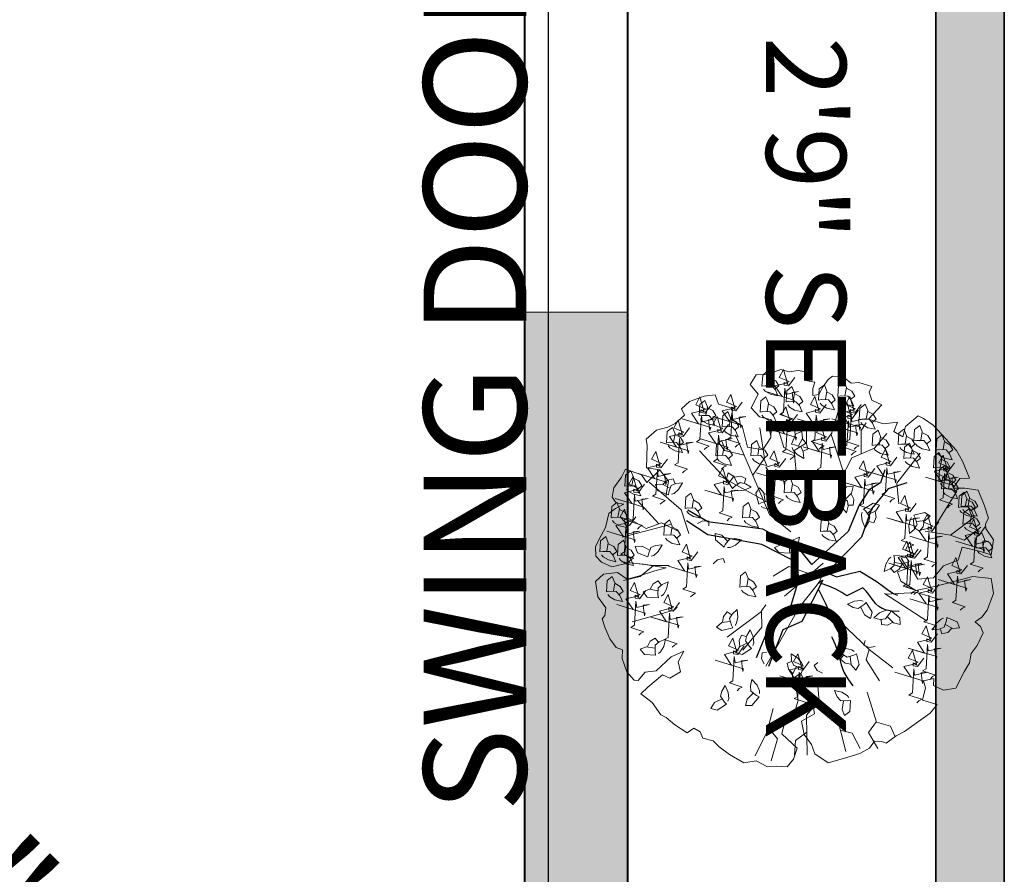
# Model space of a CAD drawing. Units: inches. Extents: x 2337 to 3570, y 1258 to 1938.
# Tile 26 of 30: x 3382 to 3468, y 1598 to 1673. Entities that reach past the tile are written whole.
import ezdxf

# ---------------------------------------------------------------- set-up
doc = ezdxf.new("R2010")
doc.units = ezdxf.units.IN
for name, color, linetype, lineweight in [('A-ANNO-DIMS', 2, 'Continuous', 18), ('A-ANNO-TEXT', 7, 'Continuous', 18), ('A-GLAZ', 4, 'Continuous', 18), ('A-WALL', 7, 'Continuous', 40), ('ARBOL', 74, 'Continuous', 13), ('C-PROP', 7, 'Continuous', 35)]:
    doc.layers.add(name, color=color, linetype=linetype, lineweight=lineweight)
doc.layers.add('A-WALL-PATT', color=18, linetype='Continuous', lineweight=13, true_color=0x000000)
doc.layers.add('C-PROP-PATT', color=251, linetype='Continuous', lineweight=13, true_color=0x636466)
doc.layers.add('TALLO', color=36, linetype='Continuous')
doc.styles.get("Standard").update_dxf_attribs({"font": 'arial.ttf'})
doc.dimstyles.new('ISO-25', dxfattribs={"dimtxt": 9, "dimasz": 2.5, "dimexe": 1.25, "dimexo": 0.625, "dimtad": 1, "dimdec": 1, "dimlunit": 3, "dimtxsty": 'Standard', "dimcen": 2.5, "dimadec": 0, "dimazin": 0, "dimtfac": 1, "dimtdec": 1, "dimtmove": 0, "dimatfit": 3, "dimfxl": 1, "dimarcsym": 0})

# ---------------------------------------------------------------- blocks, each defined once
blk = doc.blocks.new('fresno')
at = {"layer": 'ARBOL'}
for p, q in [((2.96, 0.991), (3.575, 1.984)), ((-3.638, 1.194), (-4.164, 1.76)), ((-1.151, -0.932), (-1.99, -1.556)), ((-0.974, -3.757), (-1.31, -4.423))]:
    blk.add_line(p, q, dxfattribs=at)
blk.add_lwpolyline([(0.823, 4.745), (0.566, 4.764), (0.459, 4.687), (0.336, 4.518), (0.233, 4.322), (0.087, 4.298), (0.091, 4.464), (0.14, 4.621), (-0.09, 4.659), (-0.033, 4.863), (-0.264, 4.901), (-0.483, 4.866), (-0.686, 4.924), (-1.021, 4.801), (-1.288, 4.8), (-1.431, 4.563), (-1.234, 4.327), (-1.406, 4), (-1.205, 3.778), (-0.909, 3.705), (-0.931, 3.283), (-1.122, 2.983), (-1.491, 3.043), (-1.619, 3.562), (-1.9, 3.727), (-1.851, 3.982), (-2.197, 4.084), (-2.278, 4.31), (-2.543, 4.283), (-2.896, 4.152), (-3.091, 3.971), (-3.022, 3.817), (-3.244, 3.617), (-3.424, 3.528), (-3.697, 3.455), (-3.946, 3.236), (-3.922, 3.09), (-3.94, 2.548), (-3.617, 2.495), (-3.927, 2.19), (-4.062, 2.379), (-4.443, 2.512), (-4.546, 2.316), (-4.73, 2.062), (-4.767, 1.832), (-4.671, 1.698), (-4.486, 1.667), (-4.693, 1.559), (-4.854, 1.444), (-4.934, 1.102), (-5.037, 0.905), (-5.175, 0.644), (-5.166, 0.406), (-5.024, 0.264), (-4.781, 0.153), (-4.363, 0.249), (-4.014, 0.215), (-3.783, 0.177), (-3.46, 0.124), (-3.733, 0.051), (-4.132, -0.073), (-4.404, -0.146), (-4.639, 0.011), (-4.977, -0.028), (-5.172, -0.209), (-5.113, -0.574), (-4.921, -0.843), (-4.951, -1.027), (-5.012, -1.112), (-4.95, -1.311), (-4.83, -1.592), (-4.676, -1.807), (-4.518, -1.856), (-4.529, -2.068), (-4.417, -2.394), (-4.236, -2.59), (-4.143, -2.605), (-3.967, -2.397), (-3.703, -2.37), (-3.339, -2.027), (-3.032, -1.889), (-3.169, -2.15), (-3.115, -2.396), (-3.376, -2.542), (-3.552, -2.466), (-3.909, -2.762), (-4.077, -2.924), (-3.804, -3.135), (-3.592, -3.43), (-3.461, -3.499), (-3.253, -3.676), (-2.953, -3.867), (-2.792, -3.752), (-2.642, -3.848), (-2.572, -4.001), (-2.323, -4.066), (-2.18, -4.208), (-1.926, -4.392), (-1.58, -4.591), (-1.288, -4.545), (-1.027, -4.683), (-0.788, -4.675), (-0.531, -4.693), (-0.382, -4.505), (-0.29, -4.236), (-0.66, -3.891), (-0.588, -3.595), (-0.374, -3.441), (-0.267, -3.079), (-0.368, -2.541), (-0.208, -2.426), (-0.099, -2.633), (-0.087, -2.991), (0.071, -3.04), (0.129, -3.405), (-0.185, -3.59), (-0.119, -3.909), (0.055, -4.151), (0.136, -4.377), (0.456, -4.596), (0.828, -4.491), (1.227, -4.368), (1.461, -4.241), (1.583, -4.071), (1.748, -4.075), (1.86, -4.117), (2.101, -3.944), (2.308, -3.836), (2.925, -3.393), (3.101, -3.185), (2.74, -3.078), (2.812, -2.782), (2.769, -2.61), (3.015, -2.555), (3.012, -2.721), (3.254, -2.832), (3.546, -2.785), (3.752, -2.393), (3.882, -2.177), (3.92, -1.947), (4.069, -1.758), (4.214, -1.451), (4.144, -1.297), (4.021, -1.182), (4.182, -1.067), (4.304, -0.897), (4.464, -0.497), (4.429, -0.279), (4.406, -0.133), (3.964, -0.083), (3.074, -0.315), (2.582, -0.424), (2.217, -0.197), (2.136, 0.029), (2.462, 0.141), (2.628, -0.147), (3.012, -0.116), (3.249, 0.177), (3.602, 0.308), (3.701, 0.623), (4.089, 0.535), (4.404, 0.436), (4.464, 0.805), (4.272, 1.074), (4.267, 1.193), (4.336, 1.324), (4.243, 1.623), (4.092, 2.003), (3.769, 2.057), (3.485, 2.056), (3.642, 2.291), (3.88, 2.299), (3.71, 2.706), (3.563, 2.967), (3.201, 3.358), (3.001, 3.581), (2.766, 3.738), (2.635, 3.807), (2.332, 3.549), (2.268, 3.299), (2.052, 3.429), (2.136, 3.652), (1.798, 3.613), (1.437, 3.72), (1.755, 4.071), (1.513, 4.182), (1.451, 4.381), (1.519, 4.512), (1.204, 4.611), (1.012, 4.596)], close=True, dxfattribs=at)
for points in [[(-1.104, 4.45), (-1.063, 4.399), (-0.939, 4.325), (-0.757, 4.285), (-0.82, 4.431), (-0.903, 4.527), (-1.075, 4.533), (-1.143, 4.521), (-1.126, 4.792), (-1.002, 4.891), (-0.939, 4.738), (-0.975, 4.535)], [(-0.346, 4.735), (-0.501, 4.528), (-0.605, 4.545), (-0.605, 4.614), (-0.519, 4.563), (-0.622, 4.925), (-0.726, 4.735), (-0.484, 4.632), (-0.622, 4.58), (-0.829, 4.528), (-0.657, 4.27), (-1.053, 4.39), (-0.363, 4.183), (-0.381, 4.114), (-0.415, 4.373), (-0.26, 4.39), (-0.57, 4.321), (-0.588, 4.476), (-0.622, 3.89), (-0.708, 3.839), (-0.398, 3.735), (-0.467, 3.701), (-0.519, 3.649)], [(-0.935, 4.717), (-0.809, 4.65), (-0.736, 4.529), (-0.824, 4.459)], [(0.263, 4.114), (0.304, 4.063), (0.429, 3.989), (0.611, 3.948), (0.547, 4.095), (0.465, 4.191), (0.293, 4.197), (0.225, 4.185), (0.242, 4.456), (0.366, 4.555), (0.428, 4.402), (0.393, 4.199)], [(0.734, 4.203), (0.775, 4.152), (0.9, 4.078), (1.082, 4.038), (1.018, 4.185), (0.936, 4.281), (0.763, 4.287), (0.696, 4.274), (0.712, 4.546), (0.837, 4.645), (0.899, 4.491), (0.863, 4.289)], [(-1.623, 4.132), (-1.778, 3.925), (-1.882, 3.942), (-1.882, 4.011), (-1.795, 3.959), (-1.899, 4.321), (-2.002, 4.132), (-1.761, 4.028), (-1.899, 3.977), (-2.106, 3.925), (-1.933, 3.666), (-2.33, 3.787), (-1.64, 3.58), (-1.657, 3.511), (-1.692, 3.77), (-1.537, 3.787), (-1.847, 3.718), (-1.864, 3.873), (-1.899, 3.287), (-1.985, 3.235), (-1.675, 3.132), (-1.744, 3.097), (-1.795, 3.046)], [(-0.521, 4.069), (-0.48, 4.018), (-0.356, 3.944), (-0.174, 3.904), (-0.237, 4.051), (-0.32, 4.146), (-0.492, 4.152), (-0.56, 4.14), (-0.543, 4.411), (-0.419, 4.511), (-0.356, 4.357), (-0.392, 4.154)], [(-0.352, 4.337), (-0.226, 4.269), (-0.153, 4.148), (-0.241, 4.078)], [(0.433, 4.381), (0.558, 4.314), (0.631, 4.193), (0.544, 4.122)], [(0.904, 4.471), (1.029, 4.404), (1.102, 4.282), (1.015, 4.212)], [(-2.368, 4.073), (-2.523, 3.866), (-2.627, 3.883), (-2.627, 3.952), (-2.541, 3.9), (-2.644, 4.262), (-2.748, 4.073), (-2.506, 3.969), (-2.644, 3.918), (-2.851, 3.866), (-2.679, 3.607), (-3.075, 3.728), (-2.385, 3.521), (-2.403, 3.452), (-2.437, 3.711), (-2.282, 3.728), (-2.592, 3.659), (-2.61, 3.814), (-2.644, 3.228), (-2.73, 3.176), (-2.42, 3.073), (-2.489, 3.038), (-2.541, 2.987)], [(-2.629, 3.733), (-2.588, 3.682), (-2.463, 3.608), (-2.281, 3.568), (-2.345, 3.715), (-2.427, 3.81), (-2.6, 3.816), (-2.667, 3.804), (-2.651, 4.075), (-2.526, 4.175), (-2.464, 4.021), (-2.5, 3.818)], [(-1.149, 3.822), (-1.108, 3.771), (-0.983, 3.697), (-0.802, 3.657), (-0.865, 3.804), (-0.948, 3.9), (-1.12, 3.906), (-1.188, 3.893), (-1.171, 4.165), (-1.047, 4.264), (-0.984, 4.111), (-1.02, 3.908)], [(-0.98, 4.09), (-0.854, 4.023), (-0.781, 3.901), (-0.869, 3.831)], [(0.413, 4.08), (0.258, 3.873), (0.154, 3.89), (0.154, 3.959), (0.241, 3.908), (0.137, 4.27), (0.034, 4.08), (0.275, 3.977), (0.137, 3.925), (-0.07, 3.873), (0.103, 3.614), (-0.294, 3.735), (0.396, 3.528), (0.379, 3.459), (0.344, 3.718), (0.499, 3.735), (0.189, 3.666), (0.172, 3.821), (0.137, 3.235), (0.051, 3.183), (0.361, 3.08), (0.292, 3.046), (0.241, 2.994)], [(1.189, 3.942), (1.034, 3.735), (0.931, 3.752), (0.931, 3.821), (1.017, 3.77), (0.913, 4.132), (0.81, 3.942), (1.051, 3.839), (0.913, 3.787), (0.706, 3.735), (0.879, 3.477), (0.482, 3.597), (1.172, 3.39), (1.155, 3.321), (1.12, 3.58), (1.276, 3.597), (0.965, 3.528), (0.948, 3.683), (0.913, 3.097), (0.827, 3.046), (1.138, 2.942), (1.069, 2.908), (1.017, 2.856)], [(1.259, 4.08), (1.103, 3.873), (1, 3.89), (1, 3.959), (1.086, 3.908), (0.982, 4.27), (0.879, 4.08), (1.12, 3.977), (0.982, 3.925), (0.775, 3.873), (0.948, 3.614), (0.551, 3.735), (1.241, 3.528), (1.224, 3.459), (1.189, 3.718), (1.345, 3.735), (1.034, 3.666), (1.017, 3.821), (0.982, 3.235), (0.896, 3.183), (1.207, 3.08), (1.138, 3.046), (1.086, 2.994)], [(1.25, 3.643), (1.291, 3.592), (1.416, 3.518), (1.597, 3.478), (1.534, 3.625), (1.451, 3.721), (1.279, 3.727), (1.211, 3.714), (1.228, 3.985), (1.352, 4.085), (1.415, 3.931), (1.379, 3.729)], [(-2.459, 4), (-2.334, 3.933), (-2.261, 3.812), (-2.348, 3.742)], [(-2.068, 3.464), (-2.027, 3.413), (-1.903, 3.339), (-1.721, 3.299), (-1.784, 3.446), (-1.867, 3.542), (-2.039, 3.547), (-2.107, 3.535), (-2.09, 3.806), (-1.966, 3.906), (-1.903, 3.752), (-1.939, 3.55)], [(-0.287, 3.833), (-0.442, 3.626), (-0.546, 3.643), (-0.546, 3.712), (-0.46, 3.661), (-0.563, 4.023), (-0.667, 3.833), (-0.425, 3.73), (-0.563, 3.678), (-0.77, 3.626), (-0.598, 3.367), (-0.995, 3.488), (-0.304, 3.281), (-0.322, 3.212), (-0.356, 3.471), (-0.201, 3.488), (-0.511, 3.419), (-0.529, 3.574), (-0.563, 2.988), (-0.649, 2.936), (-0.339, 2.833), (-0.408, 2.799), (-0.46, 2.747)], [(0.837, 2.414), (0.533, 3.352), (0.697, 3.906)], [(1.419, 3.911), (1.545, 3.844), (1.618, 3.722), (1.53, 3.652)], [(-2.898, 3.511), (-3.053, 3.304), (-3.157, 3.321), (-3.157, 3.39), (-3.071, 3.339), (-3.174, 3.701), (-3.278, 3.511), (-3.036, 3.408), (-3.174, 3.356), (-3.381, 3.304), (-3.209, 3.046), (-3.605, 3.166), (-2.915, 2.959), (-2.932, 2.89), (-2.967, 3.149), (-2.812, 3.166), (-3.122, 3.097), (-3.14, 3.253), (-3.174, 2.666), (-3.26, 2.615), (-2.95, 2.511), (-3.019, 2.477), (-3.071, 2.425)], [(-1.951, 3.597), (-2.106, 3.39), (-2.209, 3.408), (-2.209, 3.477), (-2.123, 3.425), (-2.227, 3.787), (-2.33, 3.597), (-2.089, 3.494), (-2.227, 3.442), (-2.434, 3.39), (-2.261, 3.132), (-2.658, 3.252), (-1.968, 3.046), (-1.985, 2.977), (-2.02, 3.235), (-1.864, 3.252), (-2.175, 3.183), (-2.192, 3.339), (-2.227, 2.752), (-2.313, 2.701), (-2.002, 2.597), (-2.071, 2.563), (-2.123, 2.511)], [(-1.899, 3.732), (-1.773, 3.664), (-1.7, 3.543), (-1.788, 3.473)], [(-0.358, 2.895), (-0.615, 3.037), (-0.783, 3.596)], [(-0.063, 3.671), (-0.069, 3.151), (-0.364, 2.965), (-0.319, 2.449)], [(0.558, 3.402), (0.403, 3.195), (0.299, 3.212), (0.299, 3.281), (0.386, 3.23), (0.282, 3.592), (0.179, 3.402), (0.42, 3.299), (0.282, 3.247), (0.075, 3.195), (0.248, 2.936), (-0.149, 3.057), (0.541, 2.85), (0.524, 2.781), (0.489, 3.04), (0.644, 3.057), (0.334, 2.988), (0.317, 3.143), (0.282, 2.557), (0.196, 2.505), (0.506, 2.402), (0.437, 2.368), (0.386, 2.316)], [(1.259, 2.882), (1.254, 3.446), (1.381, 3.636)], [(-3.413, 3.083), (-3.373, 3.032), (-3.248, 2.958), (-3.066, 2.918), (-3.129, 3.065), (-3.212, 3.161), (-3.384, 3.167), (-3.452, 3.154), (-3.435, 3.425), (-3.311, 3.525), (-3.248, 3.371), (-3.284, 3.169)], [(-3.244, 3.351), (-3.118, 3.284), (-3.045, 3.162), (-3.133, 3.092)], [(-0.448, 1), (-0.961, 1.419), (-1.784, 3.341)], [(-1.367, 2.367), (-1.081, 2.78), (-1.193, 3.514)], [(-0.923, 3.449), (-0.951, 3.425), (-0.93, 3.313)], [(-0.41, 3.035), (-0.387, 2.974), (-0.291, 2.865), (-0.131, 2.771), (-0.146, 2.93), (-0.195, 3.047), (-0.357, 3.106), (-0.425, 3.115), (-0.325, 3.368), (-0.176, 3.424), (-0.164, 3.258), (-0.261, 3.077)], [(0.746, 2.242), (1.034, 2.786), (1.584, 3.019), (1.879, 3.374)], [(1.564, 3.016), (1.605, 2.965), (1.729, 2.891), (1.911, 2.851), (1.848, 2.998), (1.765, 3.094), (1.593, 3.099), (1.525, 3.087), (1.542, 3.358), (1.666, 3.458), (1.729, 3.304), (1.693, 3.102)], [(2.191, 3.038), (2.232, 2.987), (2.357, 2.913), (2.539, 2.873), (2.475, 3.02), (2.393, 3.116), (2.221, 3.122), (2.153, 3.109), (2.17, 3.381), (2.294, 3.48), (2.356, 3.326), (2.321, 3.124)], [(2.573, 3.128), (2.613, 3.077), (2.738, 3.003), (2.92, 2.963), (2.857, 3.11), (2.774, 3.205), (2.602, 3.211), (2.534, 3.199), (2.551, 3.47), (2.675, 3.57), (2.738, 3.416), (2.702, 3.214)], [(2.742, 3.396), (2.868, 3.328), (2.941, 3.207), (2.853, 3.137)], [(3.111, 2.904), (3.152, 2.853), (3.276, 2.779), (3.458, 2.739), (3.395, 2.886), (3.312, 2.981), (3.14, 2.987), (3.072, 2.975), (3.089, 3.246), (3.213, 3.346), (3.276, 3.192), (3.24, 2.99)], [(-2.225, 2.77), (-2.184, 2.718), (-2.06, 2.645), (-1.878, 2.604), (-1.941, 2.751), (-2.024, 2.847), (-2.196, 2.853), (-2.264, 2.84), (-2.247, 3.112), (-2.123, 3.211), (-2.06, 3.058), (-2.096, 2.855)], [(-1.575, 2.854), (-2.052, 2.969), (-2.2, 3.178)], [(-1.373, 2.77), (-1.332, 2.718), (-1.208, 2.645), (-1.026, 2.604), (-1.089, 2.751), (-1.172, 2.847), (-1.344, 2.853), (-1.412, 2.84), (-1.395, 3.112), (-1.271, 3.211), (-1.208, 3.058), (-1.244, 2.855)], [(-0.166, 3.238), (-0.068, 3.135), (-0.036, 2.997), (-0.141, 2.957)], [(1.733, 3.284), (1.859, 3.216), (1.932, 3.095), (1.844, 3.025)], [(2.326, 2.702), (2.367, 2.651), (2.492, 2.577), (2.673, 2.537), (2.61, 2.684), (2.527, 2.78), (2.355, 2.786), (2.287, 2.773), (2.304, 3.045), (2.428, 3.144), (2.491, 2.99), (2.455, 2.788)], [(2.361, 3.306), (2.486, 3.239), (2.559, 3.117), (2.472, 3.047)], [(3.28, 3.172), (3.406, 3.104), (3.479, 2.983), (3.391, 2.913)], [(-3.434, 2.752), (-3.59, 2.546), (-3.693, 2.563), (-3.693, 2.632), (-3.607, 2.58), (-3.71, 2.942), (-3.814, 2.752), (-3.572, 2.649), (-3.71, 2.597), (-3.917, 2.546), (-3.745, 2.287), (-4.142, 2.408), (-3.452, 2.201), (-3.469, 2.132), (-3.503, 2.39), (-3.348, 2.408), (-3.659, 2.339), (-3.676, 2.494), (-3.71, 1.908), (-3.797, 1.856), (-3.486, 1.753), (-3.555, 1.718), (-3.607, 1.666)], [(-1.112, 1.773), (-2.014, 2.265), (-2.654, 2.957)], [(-2.056, 3.037), (-1.93, 2.97), (-1.857, 2.849), (-1.945, 2.778)], [(-0.57, 2.77), (-0.726, 2.563), (-0.829, 2.58), (-0.829, 2.649), (-0.743, 2.597), (-0.846, 2.959), (-0.95, 2.77), (-0.708, 2.666), (-0.846, 2.615), (-1.053, 2.563), (-0.881, 2.304), (-1.278, 2.425), (-0.588, 2.218), (-0.605, 2.149), (-0.639, 2.408), (-0.484, 2.425), (-0.795, 2.356), (-0.812, 2.511), (-0.846, 1.925), (-0.933, 1.873), (-0.622, 1.77), (-0.691, 1.735), (-0.743, 1.684)], [(-1.204, 3.037), (-1.078, 2.97), (-1.005, 2.849), (-1.093, 2.778)], [(2.121, 2.804), (1.966, 2.597), (1.862, 2.615), (1.862, 2.683), (1.949, 2.632), (1.845, 2.994), (1.742, 2.804), (1.983, 2.701), (1.845, 2.649), (1.638, 2.597), (1.811, 2.339), (1.414, 2.459), (2.104, 2.252), (2.087, 2.184), (2.052, 2.442), (2.207, 2.459), (1.897, 2.39), (1.88, 2.546), (1.845, 1.959), (1.759, 1.908), (2.069, 1.804), (2, 1.77), (1.949, 1.718)], [(2.171, 1.674), (2.121, 2.172), (2.689, 2.898)], [(2.495, 2.97), (2.621, 2.903), (2.694, 2.781), (2.606, 2.711)], [(3.043, 2.478), (3.084, 2.427), (3.209, 2.353), (3.391, 2.313), (3.327, 2.46), (3.245, 2.556), (3.073, 2.562), (3.005, 2.549), (3.022, 2.82), (3.146, 2.92), (3.208, 2.766), (3.173, 2.564)], [(1.586, 2.528), (1.431, 2.321), (1.327, 2.339), (1.327, 2.408), (1.414, 2.356), (1.31, 2.718), (1.207, 2.528), (1.448, 2.425), (1.31, 2.373), (1.103, 2.321), (1.276, 2.063), (0.879, 2.184), (1.569, 1.977), (1.552, 1.908), (1.517, 2.166), (1.673, 2.184), (1.362, 2.115), (1.345, 2.27), (1.31, 1.684), (1.224, 1.632), (1.535, 1.528), (1.466, 1.494), (1.414, 1.442)], [(3.519, 2.666), (3.363, 2.459), (3.26, 2.477), (3.26, 2.546), (3.346, 2.494), (3.243, 2.856), (3.139, 2.666), (3.381, 2.563), (3.243, 2.511), (3.036, 2.459), (3.208, 2.201), (2.811, 2.321), (3.501, 2.115), (3.484, 2.046), (3.45, 2.304), (3.605, 2.321), (3.294, 2.252), (3.277, 2.408), (3.243, 1.821), (3.156, 1.77), (3.467, 1.666), (3.398, 1.632), (3.346, 1.58)], [(3.213, 2.746), (3.338, 2.679), (3.411, 2.557), (3.324, 2.487)], [(-4.422, 2.03), (-4.381, 1.979), (-4.257, 1.905), (-4.075, 1.865), (-4.138, 2.012), (-4.221, 2.108), (-4.393, 2.114), (-4.461, 2.101), (-4.444, 2.372), (-4.32, 2.472), (-4.257, 2.318), (-4.293, 2.116)], [(-3.468, 1.85), (-3.409, 2.222), (-3.628, 2.505)], [(-1.817, 2.351), (-1.972, 2.144), (-2.075, 2.162), (-2.075, 2.231), (-1.989, 2.179), (-2.093, 2.541), (-2.196, 2.351), (-1.955, 2.248), (-2.093, 2.196), (-2.3, 2.144), (-2.127, 1.886), (-2.524, 2.006), (-1.834, 1.8), (-1.851, 1.731), (-1.886, 1.989), (-1.73, 2.006), (-2.041, 1.937), (-2.058, 2.093), (-2.093, 1.506), (-2.179, 1.455), (-1.868, 1.351), (-1.937, 1.317), (-1.989, 1.265)], [(-1.786, 2.007), (-1.722, 1.99), (-1.578, 2.003), (-1.407, 2.078), (-1.545, 2.159), (-1.668, 2.188), (-1.811, 2.092), (-1.859, 2.042), (-2.004, 2.271), (-1.962, 2.425), (-1.821, 2.337), (-1.731, 2.152)], [(3.178, 2.165), (3.219, 2.113), (3.344, 2.04), (3.525, 1.999), (3.462, 2.146), (3.379, 2.242), (3.207, 2.248), (3.139, 2.236), (3.156, 2.507), (3.28, 2.606), (3.343, 2.453), (3.307, 2.25)], [(3.245, 1.963), (3.286, 1.912), (3.411, 1.838), (3.593, 1.798), (3.529, 1.945), (3.447, 2.041), (3.274, 2.046), (3.206, 2.034), (3.223, 2.305), (3.347, 2.405), (3.41, 2.251), (3.374, 2.049)], [(3.347, 2.432), (3.473, 2.365), (3.546, 2.244), (3.458, 2.173)], [(-3.986, 2.149), (-4.142, 1.942), (-4.245, 1.959), (-4.245, 2.028), (-4.159, 1.977), (-4.262, 2.339), (-4.366, 2.149), (-4.124, 2.046), (-4.262, 1.994), (-4.47, 1.942), (-4.297, 1.684), (-4.694, 1.804), (-4.004, 1.597), (-4.021, 1.528), (-4.055, 1.787), (-3.9, 1.804), (-4.211, 1.735), (-4.228, 1.89), (-4.262, 1.304), (-4.349, 1.253), (-4.038, 1.149), (-4.107, 1.115), (-4.159, 1.063)], [(-4.253, 2.298), (-4.127, 2.231), (-4.054, 2.109), (-4.142, 2.039)], [(-2.916, 0.958), (-3.096, 1.528), (-3.871, 2.197)], [(-3.331, 1.905), (-3.269, 1.928), (-3.161, 2.024), (-3.066, 2.184), (-3.226, 2.169), (-3.342, 2.121), (-3.401, 1.958), (-3.41, 1.89), (-3.663, 1.99), (-3.719, 2.139), (-3.554, 2.151), (-3.372, 2.054)], [(-3.533, 2.149), (-3.43, 2.247), (-3.292, 2.279), (-3.252, 2.174)], [(-1.806, 2.323), (-1.665, 2.343), (-1.534, 2.287), (-1.564, 2.179)], [(-0.566, 1.873), (-0.525, 1.822), (-0.4, 1.748), (-0.219, 1.708), (-0.282, 1.855), (-0.365, 1.951), (-0.537, 1.957), (-0.605, 1.944), (-0.588, 2.216), (-0.464, 2.315), (-0.401, 2.162), (-0.437, 1.959)], [(3.415, 2.231), (3.54, 2.163), (3.613, 2.042), (3.525, 1.972)], [(-2.965, 1.493), (-2.924, 1.441), (-2.799, 1.368), (-2.618, 1.327), (-2.681, 1.474), (-2.764, 1.57), (-2.936, 1.576), (-3.004, 1.564), (-2.987, 1.835), (-2.863, 1.934), (-2.8, 1.781), (-2.836, 1.578)], [(-1.164, 1.612), (-1.109, 1.576), (-0.967, 1.544), (-0.782, 1.562), (-0.888, 1.682), (-0.996, 1.748), (-1.162, 1.7), (-1.222, 1.667), (-1.29, 1.93), (-1.203, 2.063), (-1.096, 1.937), (-1.067, 1.733)], [(-1.085, 1.919), (-0.945, 1.893), (-0.838, 1.801), (-0.9, 1.707)], [(-0.397, 2.141), (-0.271, 2.074), (-0.198, 1.952), (-0.286, 1.882)], [(0.72, 1.798), (0.723, 1.733), (0.781, 1.6), (0.904, 1.46), (0.939, 1.616), (0.929, 1.742), (0.793, 1.848), (0.73, 1.878), (0.904, 2.088), (1.062, 2.095), (1.023, 1.934), (0.875, 1.791)], [(1.014, 1.915), (1.077, 1.787), (1.064, 1.646), (0.952, 1.64)], [(3.649, 1.515), (3.69, 1.464), (3.814, 1.39), (3.996, 1.35), (3.933, 1.497), (3.85, 1.592), (3.678, 1.598), (3.61, 1.586), (3.627, 1.857), (3.751, 1.957), (3.814, 1.803), (3.778, 1.601)], [(3.716, 1.537), (3.757, 1.486), (3.882, 1.412), (4.063, 1.372), (4, 1.519), (3.917, 1.615), (3.745, 1.621), (3.677, 1.608), (3.694, 1.88), (3.818, 1.979), (3.881, 1.825), (3.845, 1.623)], [(-4.759, 1.269), (-4.718, 1.217), (-4.593, 1.144), (-4.411, 1.103), (-4.475, 1.25), (-4.557, 1.346), (-4.729, 1.352), (-4.797, 1.339), (-4.78, 1.611), (-4.656, 1.71), (-4.594, 1.557), (-4.629, 1.354)], [(-2.796, 1.76), (-2.67, 1.693), (-2.597, 1.572), (-2.685, 1.501)], [(-1.575, 1.269), (-1.534, 1.217), (-1.409, 1.144), (-1.228, 1.103), (-1.291, 1.25), (-1.373, 1.346), (-1.546, 1.352), (-1.614, 1.339), (-1.597, 1.611), (-1.473, 1.71), (-1.41, 1.557), (-1.446, 1.354)], [(1.283, 1.469), (1.266, 1.405), (1.279, 1.261), (1.354, 1.09), (1.435, 1.228), (1.464, 1.351), (1.368, 1.494), (1.318, 1.542), (1.547, 1.687), (1.7, 1.645), (1.613, 1.504), (1.428, 1.414)], [(2.587, 1.684), (2.432, 1.477), (2.328, 1.494), (2.328, 1.563), (2.414, 1.511), (2.311, 1.873), (2.207, 1.684), (2.449, 1.58), (2.311, 1.528), (2.104, 1.477), (2.276, 1.218), (1.88, 1.339), (2.57, 1.132), (2.552, 1.063), (2.518, 1.321), (2.673, 1.339), (2.363, 1.27), (2.345, 1.425), (2.311, 0.839), (2.225, 0.787), (2.535, 0.684), (2.466, 0.649), (2.414, 0.597)], [(3.818, 1.783), (3.944, 1.715), (4.017, 1.594), (3.929, 1.524)], [(3.885, 1.805), (4.011, 1.738), (4.084, 1.616), (3.996, 1.546)], [(-4.193, 1.356), (-4.349, 1.149), (-4.452, 1.166), (-4.452, 1.235), (-4.366, 1.184), (-4.469, 1.546), (-4.573, 1.356), (-4.331, 1.253), (-4.469, 1.201), (-4.677, 1.149), (-4.504, 0.89), (-4.901, 1.011), (-4.211, 0.804), (-4.228, 0.735), (-4.262, 0.994), (-4.107, 1.011), (-4.418, 0.942), (-4.435, 1.097), (-4.469, 0.511), (-4.556, 0.459), (-4.245, 0.356), (-4.314, 0.322), (-4.366, 0.27)], [(-4.589, 1.536), (-4.464, 1.469), (-4.391, 1.348), (-4.478, 1.277)], [(-1.406, 1.536), (-1.28, 1.469), (-1.207, 1.348), (-1.295, 1.277)], [(1.599, 1.489), (1.618, 1.348), (1.563, 1.217), (1.455, 1.247)], [(2.479, 1.34), (2.443, 1.285), (2.411, 1.143), (2.429, 0.958), (2.549, 1.064), (2.615, 1.172), (2.567, 1.338), (2.534, 1.398), (2.797, 1.466), (2.93, 1.379), (2.804, 1.272), (2.6, 1.243)], [(3.761, 1.112), (3.802, 1.061), (3.926, 0.987), (4.108, 0.947), (4.045, 1.093), (3.962, 1.189), (3.79, 1.195), (3.722, 1.183), (3.739, 1.454), (3.863, 1.553), (3.926, 1.4), (3.89, 1.197)], [(-3.192, 1.017), (-3.578, 1.215), (-3.949, 1.081), (-4.398, 1.339)], [(-3.481, 0.843), (-3.44, 0.792), (-3.315, 0.718), (-3.133, 0.678), (-3.197, 0.825), (-3.279, 0.92), (-3.451, 0.926), (-3.519, 0.914), (-3.502, 1.185), (-3.378, 1.285), (-3.316, 1.131), (-3.351, 0.928)], [(-2.703, 1.201), (-2.575, 1.263), (-2.433, 1.251), (-2.428, 1.139)], [(0.308, 0.933), (0.349, 0.881), (0.474, 0.807), (0.656, 0.767), (0.592, 0.914), (0.51, 1.01), (0.337, 1.016), (0.27, 1.003), (0.286, 1.275), (0.411, 1.374), (0.473, 1.221), (0.437, 1.018)], [(0.478, 1.2), (0.603, 1.133), (0.676, 1.011), (0.589, 0.941)], [(3.139, 1.235), (2.984, 1.028), (2.88, 1.046), (2.88, 1.115), (2.967, 1.063), (2.863, 1.425), (2.759, 1.235), (3.001, 1.132), (2.863, 1.08), (2.656, 1.028), (2.828, 0.77), (2.432, 0.891), (3.122, 0.684), (3.105, 0.615), (3.07, 0.873), (3.225, 0.891), (2.915, 0.822), (2.897, 0.977), (2.863, 0.391), (2.777, 0.339), (3.087, 0.235), (3.018, 0.201), (2.967, 0.149)], [(2.786, 1.261), (2.76, 1.121), (2.668, 1.014), (2.574, 1.076)], [(4.01, 1.36), (3.422, 0.918)], [(4.26, 1.115), (4.105, 0.908), (4.002, 0.925), (4.002, 0.994), (4.088, 0.942), (3.984, 1.304), (3.881, 1.115), (4.122, 1.011), (3.984, 0.959), (3.777, 0.908), (3.95, 0.649), (3.553, 0.77), (4.243, 0.563), (4.226, 0.494), (4.191, 0.753), (4.347, 0.77), (4.036, 0.701), (4.019, 0.856), (3.984, 0.27), (3.898, 0.218), (4.209, 0.115), (4.14, 0.08), (4.088, 0.029)], [(3.93, 1.379), (4.056, 1.312), (4.129, 1.191), (4.041, 1.121)], [(-3.354, 1.176), (-4.529, 0.864)], [(-3.311, 1.111), (-3.186, 1.043), (-3.113, 0.922), (-3.2, 0.852)], [(-1.981, 0.615), (-1.915, 0.618), (-1.782, 0.676), (-1.643, 0.799), (-1.799, 0.834), (-1.925, 0.824), (-2.031, 0.688), (-2.061, 0.626), (-2.27, 0.799), (-2.278, 0.958), (-2.117, 0.918), (-1.974, 0.77)], [(2.808, 1.015), (3.422, 0.918), (3.422, 0.918), (3.748, 0.794), (4.154, 1.111)], [(4.075, 0.529), (4.116, 0.478), (4.24, 0.404), (4.422, 0.364), (4.359, 0.511), (4.276, 0.607), (4.104, 0.613), (4.036, 0.6), (4.053, 0.871), (4.177, 0.971), (4.24, 0.817), (4.204, 0.615)], [(-5.028, 0.44), (-4.987, 0.388), (-4.862, 0.315), (-4.68, 0.274), (-4.744, 0.421), (-4.826, 0.517), (-4.998, 0.523), (-5.066, 0.511), (-5.049, 0.782), (-4.925, 0.881), (-4.863, 0.728), (-4.898, 0.525)], [(-4.602, 0.35), (-4.561, 0.299), (-4.436, 0.225), (-4.254, 0.185), (-4.318, 0.332), (-4.4, 0.428), (-4.572, 0.433), (-4.64, 0.421), (-4.623, 0.692), (-4.499, 0.792), (-4.437, 0.638), (-4.472, 0.436)], [(-0.397, 0.517), (-0.346, 0.557), (-0.272, 0.682), (-0.232, 0.864), (-0.379, 0.801), (-0.474, 0.718), (-0.48, 0.546), (-0.468, 0.478), (-0.739, 0.495), (-0.838, 0.619), (-0.685, 0.682), (-0.482, 0.646)], [(2.639, 0.58), (2.483, 0.373), (2.38, 0.391), (2.38, 0.46), (2.466, 0.408), (2.363, 0.77), (2.259, 0.58), (2.501, 0.477), (2.363, 0.425), (2.156, 0.373), (2.328, 0.115), (1.931, 0.235), (2.621, 0.029), (2.604, -0.04), (2.57, 0.218), (2.725, 0.235), (2.414, 0.166), (2.397, 0.322), (2.363, -0.265), (2.276, -0.316), (2.587, -0.42), (2.518, -0.454), (2.466, -0.506)], [(2.708, 0.563), (2.552, 0.356), (2.449, 0.373), (2.449, 0.442), (2.535, 0.391), (2.432, 0.753), (2.328, 0.563), (2.57, 0.46), (2.432, 0.408), (2.225, 0.356), (2.397, 0.097), (2, 0.218), (2.69, 0.011), (2.673, -0.058), (2.639, 0.201), (2.794, 0.218), (2.483, 0.149), (2.466, 0.304), (2.432, -0.282), (2.345, -0.334), (2.656, -0.437), (2.587, -0.471), (2.535, -0.523)], [(4.244, 0.797), (4.37, 0.73), (4.443, 0.608), (4.355, 0.538)], [(-4.858, 0.707), (-4.733, 0.64), (-4.66, 0.519), (-4.747, 0.448)], [(-4.432, 0.618), (-4.307, 0.55), (-4.234, 0.429), (-4.321, 0.359)], [(-3.824, 0.404), (-3.763, 0.427), (-3.654, 0.523), (-3.559, 0.683), (-3.719, 0.668), (-3.835, 0.62), (-3.894, 0.457), (-3.903, 0.389), (-4.156, 0.489), (-4.212, 0.638), (-4.047, 0.65), (-3.865, 0.553)], [(-2.698, 0.509), (-2.854, 0.302), (-2.957, 0.319), (-2.957, 0.388), (-2.871, 0.336), (-2.974, 0.698), (-3.078, 0.509), (-2.836, 0.405), (-2.974, 0.353), (-3.182, 0.302), (-3.009, 0.043), (-3.406, 0.164), (-2.716, -0.043), (-2.733, -0.112), (-2.767, 0.147), (-2.612, 0.164), (-2.923, 0.095), (-2.94, 0.25), (-2.974, -0.336), (-3.061, -0.388), (-2.75, -0.491), (-2.819, -0.526), (-2.871, -0.577)], [(-3.394, 0.18), (-3.77, 0.182), (-4.532, 0.27)], [(-2.322, 0.222), (-2.219, 0.321), (-2.081, 0.353), (-2.042, 0.248)], [(1.978, 0.384), (1.927, 0.343), (1.853, 0.218), (1.813, 0.036), (1.96, 0.1), (2.056, 0.182), (2.061, 0.355), (2.049, 0.422), (2.32, 0.406), (2.42, 0.281), (2.266, 0.219), (2.064, 0.254)], [(3.829, 0.184), (3.674, -0.023), (3.57, -0.006), (3.57, 0.063), (3.657, 0.011), (3.553, 0.373), (3.45, 0.184), (3.691, 0.08), (3.553, 0.029), (3.346, -0.023), (3.519, -0.282), (3.122, -0.161), (3.812, -0.368), (3.795, -0.437), (3.76, -0.178), (3.915, -0.161), (3.605, -0.23), (3.588, -0.075), (3.553, -0.661), (3.467, -0.713), (3.777, -0.816), (3.708, -0.851), (3.657, -0.902)], [(-3.77, 0.182), (-4.09, -0.088), (-4.494, -0.18)], [(-1.642, -0.412), (-1.601, -0.463), (-1.477, -0.537), (-1.295, -0.577), (-1.358, -0.43), (-1.441, -0.334), (-1.613, -0.328), (-1.681, -0.341), (-1.664, -0.069), (-1.54, 0.03), (-1.477, -0.124), (-1.513, -0.326)], [(0.03, -0.026), (-0.491, 0.154), (-0.871, -0.08)], [(-0.596, -0.564), (0.03, -0.026), (0.339, 0.235)], [(0.38, 0.131), (0.248, -0.21), (-0.33, -0.951)], [(2.246, 0.214), (2.178, 0.089), (2.057, 0.016), (1.987, 0.103)], [(-4.871, -0.524), (-4.83, -0.575), (-4.705, -0.649), (-4.523, -0.689), (-4.587, -0.542), (-4.669, -0.446), (-4.841, -0.44), (-4.909, -0.453), (-4.893, -0.181), (-4.768, -0.082), (-4.706, -0.236), (-4.741, -0.438)], [(-3.952, -0.42), (-4.107, -0.627), (-4.211, -0.609), (-4.211, -0.54), (-4.124, -0.592), (-4.228, -0.23), (-4.331, -0.42), (-4.09, -0.523), (-4.228, -0.575), (-4.435, -0.627), (-4.262, -0.885), (-4.659, -0.765), (-3.969, -0.971), (-3.986, -1.04), (-4.021, -0.782), (-3.866, -0.765), (-4.176, -0.834), (-4.193, -0.678), (-4.228, -1.265), (-4.314, -1.316), (-4.004, -1.42), (-4.073, -1.454), (-4.124, -1.506)], [(-3.58, -0.559), (-3.529, -0.518), (-3.455, -0.393), (-3.415, -0.211), (-3.562, -0.275), (-3.658, -0.357), (-3.664, -0.53), (-3.651, -0.597), (-3.923, -0.581), (-4.022, -0.456), (-3.868, -0.394), (-3.666, -0.43)], [(-3.848, -0.389), (-3.781, -0.264), (-3.659, -0.191), (-3.589, -0.278)], [(-1.473, -0.144), (-1.347, -0.211), (-1.274, -0.333), (-1.362, -0.403)], [(3.139, -0.282), (2.984, -0.489), (2.88, -0.471), (2.88, -0.402), (2.967, -0.454), (2.863, -0.092), (2.759, -0.282), (3.001, -0.385), (2.863, -0.437), (2.656, -0.489), (2.828, -0.747), (2.432, -0.627), (3.122, -0.834), (3.105, -0.902), (3.07, -0.644), (3.225, -0.627), (2.915, -0.696), (2.897, -0.54), (2.863, -1.127), (2.777, -1.178), (3.087, -1.282), (3.018, -1.316), (2.967, -1.368)], [(-4.701, -0.256), (-4.576, -0.323), (-4.503, -0.445), (-4.59, -0.515)], [(1.846, -0.51), (2.605, -0.469), (3.129, -0.637)], [(-3.141, -0.713), (-3.296, -0.92), (-3.4, -0.902), (-3.4, -0.834), (-3.314, -0.885), (-3.417, -0.523), (-3.521, -0.713), (-3.279, -0.816), (-3.417, -0.868), (-3.624, -0.92), (-3.452, -1.178), (-3.848, -1.058), (-3.158, -1.265), (-3.175, -1.333), (-3.21, -1.075), (-3.055, -1.058), (-3.365, -1.127), (-3.383, -0.971), (-3.417, -1.558), (-3.503, -1.609), (-3.193, -1.713), (-3.262, -1.747), (-3.314, -1.799)], [(1.304, -0.681), (1.241, -0.664), (1.097, -0.678), (0.926, -0.752), (1.064, -0.833), (1.187, -0.862), (1.33, -0.766), (1.377, -0.716), (1.523, -0.945), (1.481, -1.099), (1.34, -1.011), (1.25, -0.826)], [(1.822, -0.495), (2.859, -1.165)], [(-3.195, -0.824), (-3.267, -0.898), (-4.285, -1.185)], [(-1.794, -1.268), (-1.758, -1.214), (-1.726, -1.072), (-1.744, -0.887), (-1.865, -0.993), (-1.93, -1.101), (-1.883, -1.266), (-1.85, -1.327), (-2.113, -1.395), (-2.246, -1.307), (-2.119, -1.2), (-1.916, -1.172)], [(-2.101, -1.19), (-2.076, -1.05), (-1.983, -0.943), (-1.889, -1.004)], [(-1.047, -0.767), (-1.151, -0.913), (-1.144, -1.307), (-1.61, -1.871)], [(1.903, -0.903), (1.837, -0.905), (1.704, -0.963), (1.565, -1.086), (1.721, -1.122), (1.847, -1.111), (1.953, -0.975), (1.983, -0.913), (2.192, -1.086), (2.2, -1.245), (2.039, -1.205), (1.896, -1.057)], [(-0.346, -1.024), (-1.05, -2.251)], [(0.748, -1.185), (1.452, -1.855), (2.021, -2.292)], [(2.02, -1.197), (1.891, -1.259), (1.75, -1.247), (1.745, -1.134)], [(3.253, -1.094), (3.192, -1.117), (3.083, -1.213), (2.988, -1.374), (3.148, -1.359), (3.264, -1.31), (3.323, -1.148), (3.332, -1.079), (3.585, -1.179), (3.641, -1.328), (3.476, -1.34), (3.294, -1.244)], [(-1.361, -1.756), (-1.343, -1.693), (-1.357, -1.548), (-1.431, -1.377), (-1.513, -1.515), (-1.542, -1.638), (-1.445, -1.781), (-1.395, -1.829), (-1.625, -1.974), (-1.778, -1.932), (-1.691, -1.791), (-1.506, -1.701)], [(3.105, -1.471), (2.949, -1.678), (2.846, -1.661), (2.846, -1.592), (2.932, -1.644), (2.829, -1.282), (2.725, -1.471), (2.967, -1.575), (2.829, -1.627), (2.621, -1.678), (2.794, -1.937), (2.397, -1.816), (3.087, -2.023), (3.07, -2.092), (3.036, -1.833), (3.191, -1.816), (2.88, -1.885), (2.863, -1.73), (2.829, -2.316), (2.742, -2.368), (3.053, -2.471), (2.984, -2.506), (2.932, -2.558)], [(3.455, -1.338), (3.352, -1.437), (3.214, -1.469), (3.175, -1.364)], [(-3.648, -1.948), (-3.596, -1.907), (-3.523, -1.782), (-3.482, -1.6), (-3.629, -1.664), (-3.725, -1.746), (-3.731, -1.919), (-3.719, -1.986), (-3.99, -1.97), (-4.089, -1.845), (-3.936, -1.783), (-3.733, -1.819)], [(-3.915, -1.778), (-3.848, -1.653), (-3.727, -1.58), (-3.656, -1.667)], [(-1.571, -1.764), (-1.726, -1.971), (-1.83, -1.954), (-1.83, -1.885), (-1.744, -1.937), (-1.847, -1.575), (-1.951, -1.764), (-1.709, -1.868), (-1.847, -1.92), (-2.054, -1.971), (-1.882, -2.23), (-2.278, -2.109), (-1.588, -2.316), (-1.605, -2.385), (-1.64, -2.127), (-1.485, -2.109), (-1.795, -2.178), (-1.813, -2.023), (-1.847, -2.609), (-1.933, -2.661), (-1.623, -2.764), (-1.692, -2.799), (-1.744, -2.851)], [(-1.677, -1.776), (-1.696, -1.635), (-1.641, -1.504), (-1.533, -1.534)], [(1.593, -1.781), (1.452, -1.801), (1.322, -1.746), (1.352, -1.637)], [(1.086, -1.899), (1.031, -1.863), (0.89, -1.831), (0.704, -1.849), (0.81, -1.969), (0.918, -2.035), (1.084, -1.987), (1.145, -1.954), (1.212, -2.218), (1.125, -2.35), (1.018, -2.224), (0.989, -2.02)], [(1.452, -1.855), (1.379, -2.105), (1.698, -2.609)], [(2.777, -2.058), (2.621, -2.264), (2.518, -2.247), (2.518, -2.178), (2.604, -2.23), (2.501, -1.868), (2.397, -2.058), (2.639, -2.161), (2.501, -2.213), (2.294, -2.264), (2.466, -2.523), (2.069, -2.402), (2.759, -2.609), (2.742, -2.678), (2.708, -2.42), (2.863, -2.402), (2.552, -2.471), (2.535, -2.316), (2.501, -2.902), (2.414, -2.954), (2.725, -3.057), (2.656, -3.092), (2.604, -3.144)], [(-1.092, -2.202), (-1.154, -2.074), (-1.142, -1.933), (-1.03, -1.928)], [(-0.001, -2.144), (-0.156, -2.351), (-0.26, -2.333), (-0.26, -2.264), (-0.174, -2.316), (-0.277, -1.954), (-0.381, -2.144), (-0.139, -2.247), (-0.277, -2.299), (-0.484, -2.351), (-0.312, -2.609), (-0.708, -2.489), (-0.018, -2.695), (-0.035, -2.764), (-0.07, -2.506), (0.085, -2.489), (-0.225, -2.558), (-0.243, -2.402), (-0.277, -2.989), (-0.363, -3.04), (-0.053, -3.144), (-0.122, -3.178), (-0.174, -3.23)], [(-0.161, -2.225), (-0.184, -2.163), (-0.28, -2.055), (-0.44, -1.96), (-0.425, -2.12), (-0.376, -2.236), (-0.214, -2.295), (-0.146, -2.304), (-0.246, -2.557), (-0.395, -2.613), (-0.407, -2.448), (-0.31, -2.266)], [(1.007, -2.206), (0.867, -2.181), (0.76, -2.088), (0.822, -1.994)], [(-0.405, -2.427), (-0.503, -2.324), (-0.535, -2.186), (-0.43, -2.146)], [(0.319, -2.428), (0.193, -2.361), (0.12, -2.239), (0.208, -2.169)], [(-1.201, -2.914), (-1.204, -2.849), (-1.262, -2.716), (-1.385, -2.576), (-1.42, -2.732), (-1.41, -2.858), (-1.274, -2.964), (-1.212, -2.994), (-1.385, -3.204), (-1.544, -3.211), (-1.504, -3.05), (-1.356, -2.907)], [(-1.966, -3.1), (-1.949, -3.037), (-1.962, -2.892), (-2.037, -2.722), (-2.118, -2.859), (-2.147, -2.982), (-2.051, -3.125), (-2.001, -3.173), (-2.23, -3.319), (-2.383, -3.277), (-2.296, -3.136), (-2.111, -3.046)], [(0.201, -2.655), (0.24, -3.105), (0.657, -3.436), (0.886, -4.322)], [(0.959, -3.012), (0.918, -2.961), (0.793, -2.887), (0.612, -2.847), (0.675, -2.994), (0.758, -3.089), (0.93, -3.095), (0.998, -3.083), (0.981, -3.354), (0.857, -3.453), (0.794, -3.3), (0.83, -3.097)], [(0.238, -3.084), (-0.067, -3.438), (-0.048, -4.412)], [(1.399, -2.886), (1.63, -3.612), (1.964, -3.708), (2.084, -3.964)], [(-0.923, -4.549), (-0.768, -4.012), (-0.99, -3.737), (-0.872, -3.28)], [(0.752, -3.801), (1.042, -3.878), (1.233, -4.25)], [(1.625, -3.596), (1.438, -3.858), (1.657, -4.248)], [(-0.059, -3.851), (-0.336, -4.054), (-0.355, -4.41)]]:
    blk.add_lwpolyline(points, dxfattribs=at)
for p in [(-0.308, 0.101), (0.124, 0.027)]:
    blk.add_point(p, dxfattribs=at)
at = {"layer": 'TALLO'}
for points in [[(1.829, 2.5), (1.722, 2.184), (1.454, 2.012), (1.213, 1.639), (0.944, 1.008), (0.06, 0.204), (-0.234, 0.577), (-1.119, 1.065), (-2.458, 1.237), (-2.941, 1.524)], [(2.364, 2.184), (1.909, 2.041), (1.507, 1.552), (1.266, 0.864), (0.542, 0.125), (0.433, 0.001), (0.662, -0.096), (1.228, 0.045), (1.455, -0.09), (1.644, -0.216), (1.8, -0.33), (1.931, -0.425), (2.042, -0.496), (2.141, -0.539)], [(-1.272, -2.047), (-0.931, -1.203), (-0.475, -0.916), (-0.234, -0.112), (-0.422, 0.318), (-1.146, 0.691), (-2.458, 0.921), (-2.967, 1.266)], [(2.177, -0.932), (2.008, -0.924), (1.873, -0.898), (1.766, -0.859), (1.682, -0.807), (1.613, -0.745), (1.554, -0.676), (1.499, -0.6), (1.442, -0.521), (1.376, -0.44), (1.298, -0.357), (0.908, -0.555), (0.791, -0.474), (0.647, -0.394), (0.474, -0.317), (0.265, -0.244), (0.226, -0.233), (0.328, -0.17), (-0.181, -1.175), (-0.637, -1.375), (-0.985, -2.265)], [(0.219, -0.386), (0.3, -0.544), (0.399, -0.753), (0.473, -0.922), (0.529, -1.057), (0.571, -1.164), (0.607, -1.251), (0.641, -1.324), (0.68, -1.389), (0.729, -1.454), (0.784, -1.525), (0.844, -1.61), (0.903, -1.717)], [(0.538, -1.536), (0.555, -1.568), (0.626, -1.728), (0.678, -1.871), (0.716, -2), (0.747, -2.115), (0.773, -2.219), (0.802, -2.314), (0.837, -2.401), (0.883, -2.483), (0.936, -2.562), (0.994, -2.642), (1.052, -2.727)]]:
    blk.add_lwpolyline(points, dxfattribs=at)
blk = doc.blocks.new('*D68')
at = {"layer": 'A-ANNO-DIMS', "color": 0, "lineweight": -2, "transparency": 16777216}
for p, q in [((3427.886, 1596.116), (3427.886, 1741.994)), ((3420.411, 1596.116), (3429.136, 1596.116)), ((3427.886, 1544.616), (3427.886, 1593.616)), ((3420.411, 1542.116), (3429.136, 1542.116))]:
    blk.add_line(p, q, dxfattribs=at)
at = {"layer": 'A-ANNO-DIMS', "color": 0, "transparency": 16777216}
for points in [[(3427.469, 1593.616), (3428.303, 1593.616), (3427.886, 1596.116)], [(3427.469, 1544.616), (3428.303, 1544.616), (3427.886, 1542.116)]]:
    blk.add_solid(points, dxfattribs=at)
at = {"layer": 'Defpoints', "color": 0, "transparency": 16777216}
for p in [(3419.786, 1596.116), (3427.886, 1596.116), (3419.786, 1542.116)]:
    blk.add_point(p, dxfattribs=at)
at = {"layer": 'A-ANNO-DIMS', "color": 0, "transparency": 16777216, "insert": (3422.605, 1670.305), "char_height": 9, "attachment_point": 5, "rotation": 90}
blk.add_mtext('SWING DOOR 4\'-6" TYP.', dxfattribs=at)
blk = doc.blocks.new('*D120')
at = {"layer": 'A-ANNO-DIMS', "color": 0, "lineweight": -2, "transparency": 16777216}
for p, q in [((3353.535, 1614.367), (3384.077, 1583.825)), ((3419.786, 1548.116), (3385.845, 1582.057))]:
    blk.add_line(p, q, dxfattribs=at)
at = {"layer": 'A-ANNO-DIMS', "color": 0, "transparency": 16777216}
blk.add_solid([(3384.372, 1584.119), (3383.783, 1583.53), (3385.845, 1582.057)], dxfattribs=at)
at = {"layer": 'Defpoints', "color": 0, "transparency": 16777216}
for p in [(3385.845, 1582.057), (3419.786, 1548.116)]:
    blk.add_point(p, dxfattribs=at)
at = {"layer": 'A-ANNO-DIMS', "color": 0, "transparency": 16777216, "insert": (3369.171, 1606.113), "char_height": 9, "attachment_point": 5, "rotation": 315.0001}
blk.add_mtext('R4\'-0"', dxfattribs=at)

msp = doc.modelspace()

# ---------------------------------------------------------------- hatches: boundary and pattern name
at = {"layer": 'A-WALL-PATT'}
h = msp.add_hatch(color=256, dxfattribs=at)
h.dxf.hatch_style = 1
h.paths.add_polyline_path([(3233.786, 1857.116), (3017.786, 1857.116), (3017.786, 1824.116), (3026.786, 1824.116), (3026.786, 1848.116), (3233.786, 1848.116)])
h.paths.add_polyline_path([(3128.786, 1764.116), (3026.786, 1764.116), (3026.786, 1788.116), (3017.786, 1788.116), (3017.786, 1743.116), (3026.786, 1743.116), (3026.786, 1755.116), (3128.786, 1755.116)])
h.paths.add_polyline_path([(3245.786, 1761.116), (3245.786, 1764.116), (3164.786, 1764.116), (3164.786, 1755.116), (3170.786, 1755.116), (3170.786, 1701.116), (3224.786, 1701.116), (3224.786, 1605.116), (3233.786, 1605.116), (3233.786, 1713.116), (3224.786, 1713.116), (3224.786, 1707.116), (3176.786, 1707.116), (3176.786, 1755.116), (3224.786, 1755.116), (3224.786, 1749.116), (3233.786, 1749.116), (3233.786, 1755.116), (3245.786, 1755.116)])
h.paths.add_polyline_path([(3026.786, 1707.116), (3017.786, 1707.116), (3017.786, 1617.116), (3026.786, 1617.116), (3026.786, 1635.116), (3068.786, 1635.116), (3068.786, 1641.116), (3026.786, 1641.116)])
h.paths.add_polyline_path([(3104.786, 1551.116), (3026.786, 1551.116), (3026.786, 1569.116), (3017.786, 1569.116), (3017.786, 1518.116), (3026.786, 1518.116), (3026.786, 1542.116), (3104.786, 1542.116)])
h.paths.add_polyline_path([(3026.786, 1482.116), (3017.786, 1482.116), (3017.786, 1410.116), (3026.786, 1410.116)])
h.paths.add_polyline_path([(3188.786, 1350.116), (3152.786, 1350.116), (3152.786, 1380.116), (3146.786, 1380.116), (3146.786, 1350.116), (3026.786, 1350.116), (3026.786, 1374.116), (3017.786, 1374.116), (3017.786, 1341.116), (3188.786, 1341.116)])
h.paths.add_polyline_path([(3224.786, 1416.116), (3248.786, 1416.116), (3248.786, 1422.116), (3152.786, 1422.116), (3152.786, 1542.116), (3242.786, 1542.116), (3242.786, 1551.116), (3233.786, 1551.116), (3233.786, 1557.116), (3224.786, 1557.116), (3224.786, 1551.116), (3140.786, 1551.116), (3140.786, 1542.116), (3146.786, 1542.116), (3146.786, 1410.116), (3152.786, 1410.116), (3152.786, 1416.116), (3218.786, 1416.116), (3218.786, 1350.116), (3212.786, 1350.116), (3212.786, 1341.116), (3293.786, 1341.116), (3293.786, 1362.116), (3284.786, 1362.116), (3284.786, 1350.116), (3224.786, 1350.116)])
h.paths.add_polyline_path([(3293.786, 1434.116), (3284.786, 1434.116), (3284.786, 1422.116), (3278.786, 1422.116), (3278.786, 1416.116), (3284.786, 1416.116), (3284.786, 1386.116), (3293.786, 1386.116)], flags=17)
h.paths.add_polyline_path([(3293.786, 1542.116), (3314.786, 1542.116), (3314.786, 1551.116), (3278.786, 1551.116), (3278.786, 1545.116), (3278.786, 1542.116), (3284.786, 1542.116), (3284.786, 1482.116), (3293.786, 1482.116)])
h.paths.add_polyline_path([(3371.786, 1551.116), (3350.786, 1551.116), (3350.786, 1542.116), (3371.786, 1542.116), (3371.786, 1548.116)])
h.paths.add_polyline_path([(3434.786, 1647.116), (3425.786, 1647.116), (3425.786, 1551.116), (3419.786, 1551.116), (3419.786, 1548.116), (3419.786, 1542.116), (3434.786, 1542.116)])
h.paths.add_polyline_path([(3434.786, 1764.116), (3389.786, 1764.116), (3389.786, 1755.116), (3425.786, 1755.116), (3425.786, 1719.116), (3434.786, 1719.116)])
h.paths.add_polyline_path([(3317.786, 1764.116), (3281.786, 1764.116), (3281.786, 1755.116), (3317.786, 1755.116)])
at = {"layer": 'C-PROP-PATT'}
h = msp.add_hatch(color=256, dxfattribs=at)
h.dxf.hatch_style = 1
h.paths.add_polyline_path([(3467.786, 1893.116), (2987.786, 1893.116), (2987.786, 1293.116), (3293.786, 1293.116), (3293.786, 1299.116), (2993.786, 1299.116), (2993.786, 1887.116), (3461.786, 1887.116), (3461.786, 1875.116), (3467.786, 1875.116)])
h.paths.add_polyline_path([(3407.786, 1299.116), (3389.786, 1299.116), (3389.786, 1293.116), (3407.786, 1293.116)], flags=17)
h.paths.add_polyline_path([(3461.786, 1299.116), (3455.786, 1299.116), (3455.786, 1293.116), (3467.786, 1293.116), (3467.786, 1779.116), (3461.786, 1779.116)], flags=17)

# ---------------------------------------------------------------- linework, layer by layer
at = {"layer": 'A-GLAZ'}
msp.add_line((3434.786, 1647.116), (3425.786, 1647.116), dxfattribs=at)
at = {"layer": 'A-WALL'}
for p, q in [((3434.786, 1764.116), (3434.786, 1542.116)), ((3425.786, 1755.116), (3425.786, 1551.116))]:
    msp.add_line(p, q, dxfattribs=at)
at = {"layer": 'C-PROP'}
for p, q in [((3461.786, 1779.116), (3461.786, 1299.116)), ((3467.786, 1779.116), (3467.786, 1293.116))]:
    msp.add_line(p, q, dxfattribs=at)

# ---------------------------------------------------------------- block references
at = {"layer": 'ARBOL', "xscale": 3.617267037020409, "yscale": 3.617267037020409, "zscale": 3.617267037020409}
msp.add_blockref('fresno', (3450.704, 1624.269), dxfattribs=at)

# ---------------------------------------------------------------- texts
at = {"layer": 'A-ANNO-TEXT', "insert": (3453.934, 1671.219), "char_height": 7, "attachment_point": 1, "rotation": 270}
msp.add_mtext_dynamic_manual_height_columns('2\'9" SETBACK', width=66.91102, gutter_width=12.5, heights=[0], dxfattribs=at)

# ---------------------------------------------------------------- dimensions: what is measured, and where the dimension line sits
at = {"layer": 'A-ANNO-DIMS'}
dim = msp.add_linear_dim(base=(3427.886, 1596.116), p1=(3419.786, 1542.116), p2=(3419.786, 1596.116), angle=90, text='SWING DOOR <> TYP.', dimstyle='ISO-25', override={"dimdec": 1, "dimlfac": 1, "dimrnd": 0, "dimzin": 1, "dimdsep": 46, "dimlunit": 4, "dimfrac": 2}, dxfattribs=at)
dim.commit()
dim.dimension.update_dxf_attribs({"geometry": '*D68', "text_midpoint": (3422.605, 1670.305)})
dim = msp.add_radius_dim(center=(3419.786, 1548.116), mpoint=(3385.845, 1582.057), dimstyle='ISO-25', override={"dimdec": 1, "dimlfac": 1, "dimrnd": 0, "dimzin": 1, "dimdsep": 46, "dimlunit": 4, "dimfrac": 2}, dxfattribs=at)
dim.commit()
dim.dimension.update_dxf_attribs({"geometry": '*D120', "text_midpoint": (3365.48, 1602.422), "dimtype": 164})

doc.saveas('drawing.dxf')
